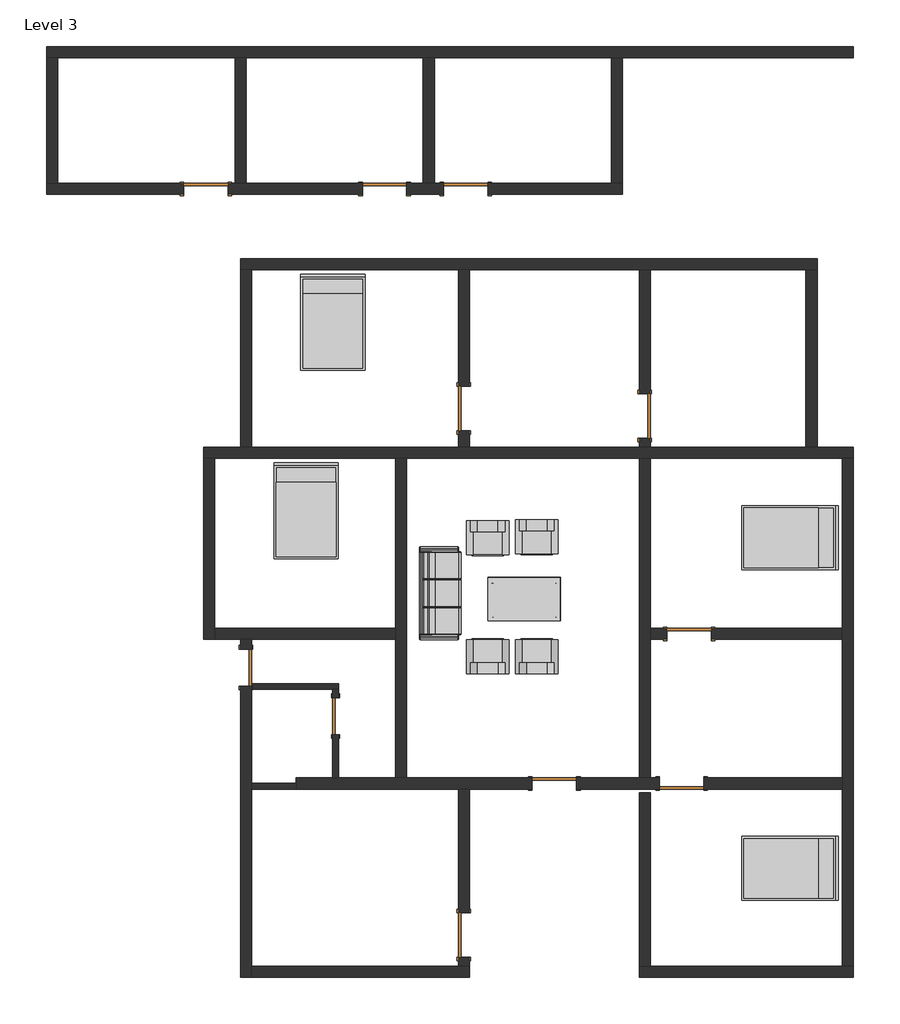
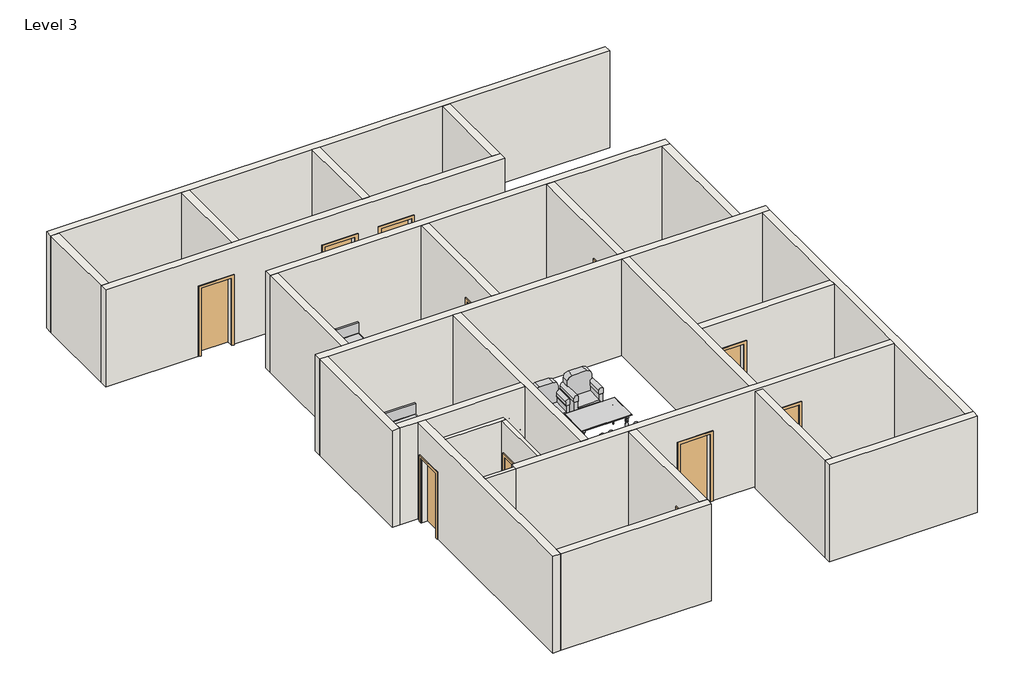
# One storey, incomplete: 27 walls, 11 doors, 10 furniture elements.
"""IFC4 building model written with IfcOpenShell, lengths in millimetres."""

from ifc_helpers import new_model, si_unit, frame, origin, place, context, project, spatial, polyline, outline, extrude, faceted_brep, transform, mapped, element, save
from components import door_a1484949, door_d8f5dbb5, door_0ca8825f, door_a90ba1ad, furniture_2fc85b74, furniture_29a9adb8, furniture_57072a26, bed_17739_bed_17739_15c61121, chair_lounge_11461_couch_0866092f, dining_table_14755_dining_table_14755_d89cb775

model = new_model("IFC4")

# Units and contexts
model_context = context("Model", 3, world=origin())
ifc_project = project(units=[si_unit("LENGTHUNIT", "METRE", prefix="MILLI")], contexts=[model_context])

# Site, building, storey
site = spatial("IfcSite", under=ifc_project)
building = spatial("IfcBuilding", under=site)
storey = spatial("IfcBuildingStorey", under=building, Name="Level 3", Elevation=3200.4)

# Doors
placement = place(None, origin())
door_shape = door_a1484949(model_context)
element("IfcDoor", 1, ObjectType="Single-Flush : 30\" x 80\"", at=placement, inside=storey, context=model_context, shape_type="MappedRepresentation", body=[
    mapped(door_shape, transform((-6124.8057305, -546.3292186, 3200.4), x_axis=(0.0, -1.0, 0.0), y_axis=(1.0, 0.0, 0.0), z_axis=(0.0, 0.0, 1.0))),
])
door_2_shape = door_d8f5dbb5(model_context)
element("IfcDoor", 2, ObjectType="Single-Flush : 30\" x 80\"", at=placement, inside=storey, context=model_context, shape_type="MappedRepresentation", body=[
    mapped(door_2_shape, transform((-4276.442132, -1546.4542186, 3200.4), x_axis=(0.0, 1.0, 0.0), y_axis=(-1.0, 0.0, 0.0), z_axis=(0.0, 0.0, 1.0))),
])
door_3_shape = door_0ca8825f(model_context)
element("IfcDoor", 3, ObjectType="Single-Flush : 36\" x 84\"", at=placement, inside=storey, context=model_context, shape_type="MappedRepresentation", body=[
    mapped(door_3_shape, transform((-6952.8959326, 9329.2722985, 3200.4), x_axis=(1.0, 0.0, 0.0), y_axis=(0.0, 1.0, 0.0), z_axis=(0.0, 0.0, 1.0))),
])
element("IfcDoor", 4, ObjectType="Single-Flush : 36\" x 84\"", at=placement, inside=storey, context=model_context, shape_type="MappedRepresentation", body=[
    mapped(door_3_shape, transform((-3267.5476203, 9329.2722985, 3200.4), x_axis=(1.0, 0.0, 0.0), y_axis=(0.0, 1.0, 0.0), z_axis=(0.0, 0.0, 1.0))),
])
element("IfcDoor", 5, ObjectType="Single-Flush : 36\" x 84\"", at=placement, inside=storey, context=model_context, shape_type="MappedRepresentation", body=[
    mapped(door_3_shape, transform((2105.307868, 4644.7957814, 3200.4), x_axis=(0.0, -1.0, 0.0), y_axis=(1.0, 0.0, 0.0), z_axis=(0.0, 0.0, 1.0))),
])
element("IfcDoor", 6, ObjectType="Single-Flush : 36\" x 84\"", at=placement, inside=storey, context=model_context, shape_type="MappedRepresentation", body=[
    mapped(door_3_shape, transform((2867.307868, -2937.1042186, 3200.4), x_axis=(-1.0, 0.0, 0.0), y_axis=(0.0, -1.0, 0.0), z_axis=(0.0, 0.0, 1.0))),
])
element("IfcDoor", 7, ObjectType="Single-Flush : 36\" x 84\"", at=placement, inside=storey, context=model_context, shape_type="MappedRepresentation", body=[
    mapped(door_3_shape, transform((238.407868, -2937.1042186, 3200.4), x_axis=(1.0, 0.0, 0.0), y_axis=(0.0, 1.0, 0.0), z_axis=(0.0, 0.0, 1.0))),
])
door_4_shape = door_a90ba1ad(model_context)
element("IfcDoor", 8, ObjectType="Single-Flush : 36\" x 84\"", at=placement, inside=storey, context=model_context, shape_type="MappedRepresentation", body=[
    mapped(door_4_shape, transform((-1591.1476203, 9329.2722985, 3200.4), x_axis=(-1.0, 0.0, 0.0), y_axis=(0.0, -1.0, 0.0), z_axis=(0.0, 0.0, 1.0))),
])
element("IfcDoor", 9, ObjectType="Single-Flush : 36\" x 84\"", at=placement, inside=storey, context=model_context, shape_type="MappedRepresentation", body=[
    mapped(door_4_shape, transform((-1628.492132, 4797.1957814, 3200.4), x_axis=(0.0, -1.0, 0.0), y_axis=(1.0, 0.0, 0.0), z_axis=(0.0, 0.0, 1.0))),
])
element("IfcDoor", 10, ObjectType="Single-Flush : 36\" x 84\"", at=placement, inside=storey, context=model_context, shape_type="MappedRepresentation", body=[
    mapped(door_4_shape, transform((3019.707868, 148.9957814, 3200.4), x_axis=(-1.0, 0.0, 0.0), y_axis=(0.0, -1.0, 0.0), z_axis=(0.0, 0.0, 1.0))),
])
element("IfcDoor", 11, ObjectType="Single-Flush : 36\" x 84\"", at=placement, inside=storey, context=model_context, shape_type="MappedRepresentation", body=[
    mapped(door_4_shape, transform((-1628.492132, -6061.3042186, 3200.4), x_axis=(0.0, -1.0, 0.0), y_axis=(1.0, 0.0, 0.0), z_axis=(0.0, 0.0, 1.0))),
])

# Furniture
furniture_shape = furniture_2fc85b74(model_context)
furniture_2_shape = furniture_29a9adb8(model_context)
furniture_3_shape = furniture_57072a26(model_context)
element("IfcFurniture", 12, at=placement, inside=storey, context=model_context, shape_type="MappedRepresentation", body=[
    mapped(furniture_shape, transform((-1742.792132, 987.1957814, 3200.4), x_axis=(0.0, 1.0, 0.0), y_axis=(-1.0, 0.0, 0.0), z_axis=(0.0, 0.0, 1.0))),
    mapped(furniture_2_shape, transform((-1742.792132, 987.1957814, 3200.4), x_axis=(0.0, 1.0, 0.0), y_axis=(-1.0, 0.0, 0.0), z_axis=(0.0, 0.0, 1.0))),
    mapped(furniture_3_shape, transform((-1742.792132, 987.1957814, 3200.4), x_axis=(0.0, 1.0, 0.0), y_axis=(-1.0, 0.0, 0.0), z_axis=(0.0, 0.0, 1.0))),
])
bed_17739_bed_17739_shape = bed_17739_bed_17739_15c61121(model_context)
element("IfcFurniture", 13, ObjectType="Bed_17739 : Bed_17739", at=placement, inside=storey, context=model_context, shape_type="MappedRepresentation", body=[
    mapped(bed_17739_bed_17739_shape, transform((-4333.592132, 6549.7957814, 3200.4), x_axis=(1.0, 0.0, 0.0), y_axis=(0.0, 1.0, 0.0), z_axis=(0.0, 0.0, 1.0))),
])
element("IfcFurniture", 14, ObjectType="Bed_17739 : Bed_17739", at=placement, inside=storey, context=model_context, shape_type="MappedRepresentation", body=[
    mapped(bed_17739_bed_17739_shape, transform((5077.107868, 2130.1957814, 3200.4), x_axis=(0.0, -1.0, 0.0), y_axis=(1.0, 0.0, 0.0), z_axis=(0.0, 0.0, 1.0))),
])
element("IfcFurniture", 15, ObjectType="Bed_17739 : Bed_17739", at=placement, inside=storey, context=model_context, shape_type="MappedRepresentation", body=[
    mapped(bed_17739_bed_17739_shape, transform((5077.107868, -4689.7042186, 3200.4), x_axis=(0.0, -1.0, 0.0), y_axis=(1.0, 0.0, 0.0), z_axis=(0.0, 0.0, 1.0))),
])
element("IfcFurniture", 16, ObjectType="Bed_17739 : Bed_17739", at=placement, inside=storey, context=model_context, shape_type="MappedRepresentation", body=[
    mapped(bed_17739_bed_17739_shape, transform((-4886.042132, 2663.5957814, 3200.4), x_axis=(1.0, 0.0, 0.0), y_axis=(0.0, 1.0, 0.0), z_axis=(0.0, 0.0, 1.0))),
])
chair_lounge_11461_couch_shape = chair_lounge_11461_couch_0866092f(model_context)
element("IfcFurniture", 17, ObjectType="Chair-Lounge_11461 : Couch", at=placement, inside=storey, context=model_context, shape_type="MappedRepresentation", body=[
    mapped(chair_lounge_11461_couch_shape, transform((-1135.6501746, 2478.1239494, 3200.4), x_axis=(1.0, 0.0, 0.0), y_axis=(0.0, 1.0, 0.0), z_axis=(0.0, 0.0, 1.0))),
])
element("IfcFurniture", 18, ObjectType="Chair-Lounge_11461 : Couch", at=placement, inside=storey, context=model_context, shape_type="MappedRepresentation", body=[
    mapped(chair_lounge_11461_couch_shape, transform((-1135.6501746, -676.3685812, 3200.4), x_axis=(-1.0, 0.0, 0.0), y_axis=(0.0, -1.0, 0.0), z_axis=(0.0, 0.0, 1.0))),
])
element("IfcFurniture", 19, ObjectType="Chair-Lounge_11461 : Couch", at=placement, inside=storey, context=model_context, shape_type="MappedRepresentation", body=[
    mapped(chair_lounge_11461_couch_shape, transform((-125.9107827, -676.3685812, 3200.4), x_axis=(-1.0, 0.0, 0.0), y_axis=(0.0, -1.0, 0.0), z_axis=(0.0, 0.0, 1.0))),
])
element("IfcFurniture", 20, ObjectType="Chair-Lounge_11461 : Couch", at=placement, inside=storey, context=model_context, shape_type="MappedRepresentation", body=[
    mapped(chair_lounge_11461_couch_shape, transform((-125.9107827, 2504.7969663, 3200.4), x_axis=(1.0, 0.0, 0.0), y_axis=(0.0, 1.0, 0.0), z_axis=(0.0, 0.0, 1.0))),
])
dining_table_14755_dining_table_14755_shape = dining_table_14755_dining_table_14755_d89cb775(model_context)
element("IfcFurniture", 21, ObjectType="Dining_table_14755 : Dining_table_14755", at=placement, inside=storey, context=model_context, shape_type="MappedRepresentation", body=[
    mapped(dining_table_14755_dining_table_14755_shape, transform((-1135.6501746, 415.6957814, 3200.4), x_axis=(1.0, 0.0, 0.0), y_axis=(0.0, 1.0, 0.0), z_axis=(0.0, 0.0, 1.0))),
])

# Walls
element("IfcWall", 22, ObjectType="4.5\"WALL", at=placement, inside=storey, context=model_context, shape_type="Brep", body=[
    faceted_brep([(-6010.5057305, -994.0042186, 3200.4), (-4333.592132, -994.0042186, 3200.4), (-4219.292132, -994.0042186, 3200.4), (-4219.292132, -994.0042186, 6248.4), (-4333.592132, -994.0042186, 6248.4), (-6010.5057305, -994.0042186, 6248.4), (-6010.5057305, -879.7042186, 3200.4), (-6010.5057305, -879.7042186, 6248.4), (-4219.292132, -879.7042186, 6248.4), (-4219.292132, -879.7042186, 3200.4)], [[[0, 1, 2, 3, 4, 5]], [[6, 7, 8, 9]], [[2, 1, 0, 6, 9]], [[0, 5, 7, 6]], [[3, 2, 9, 8]], [[5, 4, 3, 8, 7]]]),
])
element("IfcWall", 23, ObjectType="4.5\"WALL", at=placement, inside=storey, context=model_context, shape_type="SweptSolid", body=[
    extrude(outline(polyline([(-994.0042186, 3200.4), (-1165.4542186, 3200.4), (-1165.4542186, 5232.4), (-1927.4542186, 5232.4), (-1927.4542186, 3200.4), (-2822.8042186, 3200.4), (-2822.8042186, 6248.4), (-994.0042186, 6248.4), (-994.0042186, 3200.4)])), frame((-4333.592132, 0.0, 0.0), z_axis=(1.0, 0.0, 0.0), x_axis=(0.0, 1.0, 0.0)), (0.0, 0.0, 1.0), 114.3),
])
element("IfcWall", 24, ObjectType="4.5\"WALL", at=placement, inside=storey, context=model_context, shape_type="SweptSolid", body=[
    extrude(outline(polyline([(-5096.0236102, -3051.4042186), (-6010.5057305, -3051.4042186), (-6010.5057305, -2937.1042186), (-5096.0236102, -2937.1042186), (-5096.0236102, -3051.4042186)])), frame((0.0, 0.0, 3200.4), z_axis=(0.0, 0.0, 1.0), x_axis=(1.0, 0.0, 0.0)), (0.0, 0.0, 1.0), 3048.0),
])
element("IfcWall", 25, ObjectType="WALL9\"", at=placement, inside=storey, context=model_context, shape_type="Brep", body=[
    faceted_brep([(-10239.8476203, 12034.3722985, 3200.4), (-10011.2476203, 12034.3722985, 3200.4), (-6353.6476203, 12034.3722985, 3200.4), (-6125.0476203, 12034.3722985, 3200.4), (-2467.4476203, 12034.3722985, 3200.4), (-2238.8476203, 12034.3722985, 3200.4), (1418.7523797, 12034.3722985, 3200.4), (1647.3523797, 12034.3722985, 3200.4), (6410.607868, 12034.3722985, 3200.4), (6410.607868, 12034.3722985, 6248.4), (1647.3523797, 12034.3722985, 6248.4), (1418.7523797, 12034.3722985, 6248.4), (-2238.8476203, 12034.3722985, 6248.4), (-2467.4476203, 12034.3722985, 6248.4), (-6125.0476203, 12034.3722985, 6248.4), (-6353.6476203, 12034.3722985, 6248.4), (-10011.2476203, 12034.3722985, 6248.4), (-10239.8476203, 12034.3722985, 6248.4), (-10239.8476203, 12262.9722985, 3200.4), (-10239.8476203, 12262.9722985, 6248.4), (6410.607868, 12262.9722985, 6248.4), (6410.607868, 12262.9722985, 3200.4)], [[[0, 1, 2, 3, 4, 5, 6, 7, 8, 9, 10, 11, 12, 13, 14, 15, 16, 17]], [[18, 19, 20, 21]], [[8, 7, 6, 5, 4, 3, 2, 1, 0, 18, 21]], [[9, 8, 21, 20]], [[17, 16, 15, 14, 13, 12, 11, 10, 9, 20, 19]], [[0, 17, 19, 18]]]),
])
element("IfcWall", 26, ObjectType="WALL9\"", at=placement, inside=storey, context=model_context, shape_type="Brep", body=[
    faceted_brep([(-2810.3476203, 9214.9722985, 3200.4), (-2048.3476203, 9214.9722985, 3200.4), (-2048.3476203, 9214.9722985, 5334.0), (-1133.9476203, 9214.9722985, 5334.0), (-1133.9476203, 9214.9722985, 3200.4), (1647.3523797, 9214.9722985, 3200.4), (1647.3523797, 9214.9722985, 6248.4), (-6238.592132, 9214.9722985, 6248.4), (-10241.6673123, 9214.9722985, 6248.4), (-10241.6673123, 9214.9722985, 3200.4), (-7410.0959326, 9214.9722985, 3200.4), (-7410.0959326, 9214.9722985, 5334.0), (-6495.6959326, 9214.9722985, 5334.0), (-6495.6959326, 9214.9722985, 3200.4), (-3724.7476203, 9214.9722985, 3200.4), (-3724.7476203, 9214.9722985, 5334.0), (-2810.3476203, 9214.9722985, 5334.0), (-2048.3476203, 9443.5722985, 5334.0), (-2048.3476203, 9443.5722985, 3200.4), (-2238.8476203, 9443.5722985, 3200.4), (-2467.4476203, 9443.5722985, 3200.4), (-2810.3476203, 9443.5722985, 3200.4), (-2810.3476203, 9443.5722985, 5334.0), (-3724.7476203, 9443.5722985, 5334.0), (-3724.7476203, 9443.5722985, 3200.4), (-6125.0476203, 9443.5722985, 3200.4), (-6353.6476203, 9443.5722985, 3200.4), (-6495.6959326, 9443.5722985, 3200.4), (-6495.6959326, 9443.5722985, 5334.0), (-7410.0959326, 9443.5722985, 5334.0), (-7410.0959326, 9443.5722985, 3200.4), (-10011.2476203, 9443.5722985, 3200.4), (-10239.8476203, 9443.5722985, 3200.4), (-10241.6673123, 9443.5722985, 3200.4), (-10241.6673123, 9443.5722985, 6248.4), (-10239.8476203, 9443.5722985, 6248.4), (-10011.2476203, 9443.5722985, 6248.4), (-6353.6476203, 9443.5722985, 6248.4), (-6125.0476203, 9443.5722985, 6248.4), (-2467.4476203, 9443.5722985, 6248.4), (-2238.8476203, 9443.5722985, 6248.4), (1418.7523797, 9443.5722985, 6248.4), (1647.3523797, 9443.5722985, 6248.4), (1647.3523797, 9443.5722985, 3200.4), (1418.7523797, 9443.5722985, 3200.4), (-1133.9476203, 9443.5722985, 3200.4), (-1133.9476203, 9443.5722985, 5334.0)], [[[0, 1, 2, 3, 4, 5, 6, 7, 8, 9, 10, 11, 12, 13, 14, 15, 16]], [[17, 18, 19, 20, 21, 22, 23, 24, 25, 26, 27, 28, 29, 30, 31, 32, 33, 34, 35, 36, 37, 38, 39, 40, 41, 42, 43, 44, 45, 46]], [[10, 9, 33, 32, 31, 30]], [[14, 13, 27, 26, 25, 24]], [[45, 44, 43, 5, 4]], [[21, 20, 19, 18, 1, 0]], [[9, 8, 34, 33]], [[6, 5, 43, 42]], [[28, 27, 13, 12]], [[29, 28, 12, 11]], [[30, 29, 11, 10]], [[22, 21, 0, 16]], [[23, 22, 16, 15]], [[24, 23, 15, 14]], [[2, 1, 18, 17]], [[3, 2, 17, 46]], [[4, 3, 46, 45]], [[8, 7, 6, 42, 41, 40, 39, 38, 37, 36, 35, 34]]]),
])
element("IfcWall", 27, ObjectType="WALL9\"", at=placement, inside=storey, context=model_context, shape_type="SweptSolid", body=[
    extrude(outline(polyline([(1647.3523797, 12034.3722985), (1647.3523797, 9443.5722985), (1418.7523797, 9443.5722985), (1418.7523797, 12034.3722985), (1647.3523797, 12034.3722985)])), frame((0.0, 0.0, 3200.4), z_axis=(0.0, 0.0, 1.0), x_axis=(1.0, 0.0, 0.0)), (0.0, 0.0, 1.0), 3048.0),
])
element("IfcWall", 28, ObjectType="WALL9\"", at=placement, inside=storey, context=model_context, shape_type="SweptSolid", body=[
    extrude(outline(polyline([(-2467.4476203, 9443.5722985), (-2467.4476203, 12034.3722985), (-2238.8476203, 12034.3722985), (-2238.8476203, 9443.5722985), (-2467.4476203, 9443.5722985)])), frame((0.0, 0.0, 3200.4), z_axis=(0.0, 0.0, 1.0), x_axis=(1.0, 0.0, 0.0)), (0.0, 0.0, 1.0), 3048.0),
])
element("IfcWall", 29, ObjectType="WALL9\"", at=placement, inside=storey, context=model_context, shape_type="SweptSolid", body=[
    extrude(outline(polyline([(-6353.6476203, 9443.5722985), (-6353.6476203, 12034.3722985), (-6125.0476203, 12034.3722985), (-6125.0476203, 9443.5722985), (-6353.6476203, 9443.5722985)])), frame((0.0, 0.0, 3200.4), z_axis=(0.0, 0.0, 1.0), x_axis=(1.0, 0.0, 0.0)), (0.0, 0.0, 1.0), 3048.0),
])
element("IfcWall", 30, ObjectType="WALL9\"", at=placement, inside=storey, context=model_context, shape_type="Brep", body=[
    faceted_brep([(-6238.592132, 7654.6957814, 3200.4), (-6009.992132, 7654.6957814, 3200.4), (-1742.792132, 7654.6957814, 3200.4), (-1514.192132, 7654.6957814, 3200.4), (1991.007868, 7654.6957814, 3200.4), (2219.607868, 7654.6957814, 3200.4), (5432.707868, 7654.6957814, 3200.4), (5661.307868, 7654.6957814, 3200.4), (5661.307868, 7654.6957814, 6248.4), (5432.707868, 7654.6957814, 6248.4), (2219.607868, 7654.6957814, 6248.4), (1991.007868, 7654.6957814, 6248.4), (-1514.192132, 7654.6957814, 6248.4), (-1742.792132, 7654.6957814, 6248.4), (-6009.992132, 7654.6957814, 6248.4), (-6238.592132, 7654.6957814, 6248.4), (-6238.592132, 7883.2957814, 3200.4), (-6238.592132, 7883.2957814, 6248.4), (5661.307868, 7883.2957814, 6248.4), (5661.307868, 7883.2957814, 3200.4)], [[[0, 1, 2, 3, 4, 5, 6, 7, 8, 9, 10, 11, 12, 13, 14, 15]], [[16, 17, 18, 19]], [[7, 6, 5, 4, 3, 2, 1, 0, 16, 19]], [[0, 15, 17, 16]], [[15, 14, 13, 12, 11, 10, 9, 8, 18, 17]], [[8, 7, 19, 18]]]),
])
element("IfcWall", 31, ObjectType="WALL9\"", at=placement, inside=storey, context=model_context, shape_type="SweptSolid", body=[
    extrude(outline(polyline([(-6238.592132, 3997.0957814), (-6238.592132, 7654.6957814), (-6009.992132, 7654.6957814), (-6009.992132, 3997.0957814), (-6238.592132, 3997.0957814)])), frame((0.0, 0.0, 3200.4), z_axis=(0.0, 0.0, 1.0), x_axis=(1.0, 0.0, 0.0)), (0.0, 0.0, 1.0), 3048.0),
])
element("IfcWall", 32, ObjectType="WALL9\"", at=placement, inside=storey, context=model_context, shape_type="SweptSolid", body=[
    extrude(outline(polyline([(4339.9957814, 5334.0), (4339.9957814, 3200.4), (3997.0957814, 3200.4), (3997.0957814, 6248.4), (7654.6957814, 6248.4), (7654.6957814, 3200.4), (5254.3957814, 3200.4), (5254.3957814, 5334.0), (4339.9957814, 5334.0)])), frame((-1742.792132, 0.0, 0.0), z_axis=(1.0, 0.0, 0.0), x_axis=(0.0, 1.0, 0.0)), (0.0, 0.0, 1.0), 228.6),
])
element("IfcWall", 33, ObjectType="WALL9\"", at=placement, inside=storey, context=model_context, shape_type="SweptSolid", body=[
    extrude(outline(polyline([(4187.5957814, 5334.0), (4187.5957814, 3200.4), (3997.0957814, 3200.4), (3997.0957814, 6248.4), (7654.6957814, 6248.4), (7654.6957814, 3200.4), (5101.9957814, 3200.4), (5101.9957814, 5334.0), (4187.5957814, 5334.0)])), frame((1991.007868, 0.0, 0.0), z_axis=(1.0, 0.0, 0.0), x_axis=(0.0, 1.0, 0.0)), (0.0, 0.0, 1.0), 228.6),
])
element("IfcWall", 34, ObjectType="WALL9\"", at=placement, inside=storey, context=model_context, shape_type="Brep", body=[
    faceted_brep([(-7000.592132, 3768.4957814, 3200.4), (-6771.992132, 3768.4957814, 3200.4), (-3038.192132, 3768.4957814, 3200.4), (-2809.592132, 3768.4957814, 3200.4), (1991.007868, 3768.4957814, 3200.4), (2219.607868, 3768.4957814, 3200.4), (6182.007868, 3768.4957814, 3200.4), (6410.607868, 3768.4957814, 3200.4), (6410.607868, 3768.4957814, 6248.4), (6182.007868, 3768.4957814, 6248.4), (2219.607868, 3768.4957814, 6248.4), (1991.007868, 3768.4957814, 6248.4), (-2809.592132, 3768.4957814, 6248.4), (-3038.192132, 3768.4957814, 6248.4), (-6771.992132, 3768.4957814, 6248.4), (-7000.592132, 3768.4957814, 6248.4), (-7000.592132, 3997.0957814, 3200.4), (-7000.592132, 3997.0957814, 6248.4), (-6238.592132, 3997.0957814, 6248.4), (-6009.992132, 3997.0957814, 6248.4), (-1742.792132, 3997.0957814, 6248.4), (-1514.192132, 3997.0957814, 6248.4), (1991.007868, 3997.0957814, 6248.4), (2219.607868, 3997.0957814, 6248.4), (5432.707868, 3997.0957814, 6248.4), (5661.307868, 3997.0957814, 6248.4), (6410.607868, 3997.0957814, 6248.4), (6410.607868, 3997.0957814, 3200.4), (5661.307868, 3997.0957814, 3200.4), (5432.707868, 3997.0957814, 3200.4), (2219.607868, 3997.0957814, 3200.4), (1991.007868, 3997.0957814, 3200.4), (-1514.192132, 3997.0957814, 3200.4), (-1742.792132, 3997.0957814, 3200.4), (-6009.992132, 3997.0957814, 3200.4), (-6238.592132, 3997.0957814, 3200.4)], [[[0, 1, 2, 3, 4, 5, 6, 7, 8, 9, 10, 11, 12, 13, 14, 15]], [[16, 17, 18, 19, 20, 21, 22, 23, 24, 25, 26, 27, 28, 29, 30, 31, 32, 33, 34, 35]], [[7, 6, 5, 4, 3, 2, 1, 0, 16, 35, 34, 33, 32, 31, 30, 29, 28, 27]], [[0, 15, 17, 16]], [[15, 14, 13, 12, 11, 10, 9, 8, 26, 25, 24, 23, 22, 21, 20, 19, 18, 17]], [[8, 7, 27, 26]]]),
])
element("IfcWall", 35, ObjectType="WALL9\"", at=placement, inside=storey, context=model_context, shape_type="SweptSolid", body=[
    extrude(outline(polyline([(3200.4, 2219.607868), (3200.4, 2562.507868), (5334.0, 2562.507868), (5334.0, 3476.907868), (3200.4, 3476.907868), (3200.4, 6182.007868), (6248.4, 6182.007868), (6248.4, 2219.607868), (3200.4, 2219.607868)])), frame((0.0, 34.6957814, 0.0), z_axis=(0.0, 1.0, 0.0), x_axis=(0.0, 0.0, 1.0)), (0.0, 0.0, 1.0), 228.6),
])
element("IfcWall", 36, ObjectType="WALL9\"", at=placement, inside=storey, context=model_context, shape_type="Brep", body=[
    faceted_brep([(-7000.592132, 3768.4957814, 3200.4), (-7000.592132, 34.6957814, 3200.4), (-7000.592132, 34.6957814, 6248.4), (-7000.592132, 3768.4957814, 6248.4), (-6771.992132, 3768.4957814, 3200.4), (-6771.992132, 3768.4957814, 6248.4), (-6771.992132, 263.2957814, 6248.4), (-6771.992132, 34.6957814, 6248.4), (-6771.992132, 34.6957814, 3200.4), (-6771.992132, 263.2957814, 3200.4)], [[[0, 1, 2, 3]], [[4, 5, 6, 7, 8, 9]], [[1, 0, 4, 9, 8]], [[0, 3, 5, 4]], [[2, 1, 8, 7]], [[3, 2, 7, 6, 5]]]),
])
element("IfcWall", 37, ObjectType="WALL9\"", at=placement, inside=storey, context=model_context, shape_type="Brep", body=[
    faceted_brep([(-6771.992132, 34.6957814, 3200.4), (-6239.1057305, 34.6957814, 3200.4), (-6010.5057305, 34.6957814, 3200.4), (-3038.192132, 34.6957814, 3200.4), (-3038.192132, 34.6957814, 6248.4), (-6010.5057305, 34.6957814, 6248.4), (-6239.1057305, 34.6957814, 6248.4), (-6771.992132, 34.6957814, 6248.4), (-6771.992132, 263.2957814, 3200.4), (-6771.992132, 263.2957814, 6248.4), (-3038.192132, 263.2957814, 6248.4), (-3038.192132, 263.2957814, 3200.4)], [[[0, 1, 2, 3, 4, 5, 6, 7]], [[8, 9, 10, 11]], [[3, 2, 1, 0, 8, 11]], [[0, 7, 9, 8]], [[4, 3, 11, 10]], [[7, 6, 5, 4, 10, 9]]]),
])
element("IfcWall", 38, ObjectType="WALL9\"", at=placement, inside=storey, context=model_context, shape_type="Brep", body=[
    faceted_brep([(-3038.192132, 3768.4957814, 3200.4), (-3038.192132, 263.2957814, 3200.4), (-3038.192132, 34.6957814, 3200.4), (-3038.192132, -2822.8042186, 3200.4), (-3038.192132, -2822.8042186, 6248.4), (-3038.192132, 34.6957814, 6248.4), (-3038.192132, 263.2957814, 6248.4), (-3038.192132, 3768.4957814, 6248.4), (-2809.592132, 3768.4957814, 3200.4), (-2809.592132, 3768.4957814, 6248.4), (-2809.592132, -2822.8042186, 6248.4), (-2809.592132, -2822.8042186, 3200.4)], [[[0, 1, 2, 3, 4, 5, 6, 7]], [[8, 9, 10, 11]], [[3, 2, 1, 0, 8, 11]], [[0, 7, 9, 8]], [[4, 3, 11, 10]], [[7, 6, 5, 4, 10, 9]]]),
])
element("IfcWall", 39, ObjectType="WALL9\"", at=placement, inside=storey, context=model_context, shape_type="Brep", body=[
    faceted_brep([(1991.007868, 3768.4957814, 3200.4), (1991.007868, -2822.8042186, 3200.4), (1991.007868, -2822.8042186, 6248.4), (1991.007868, 3768.4957814, 6248.4), (2219.607868, 3768.4957814, 3200.4), (2219.607868, 3768.4957814, 6248.4), (2219.607868, 263.2957814, 6248.4), (2219.607868, 34.6957814, 6248.4), (2219.607868, -2822.8042186, 6248.4), (2219.607868, -2822.8042186, 3200.4), (2219.607868, 34.6957814, 3200.4), (2219.607868, 263.2957814, 3200.4)], [[[0, 1, 2, 3]], [[4, 5, 6, 7, 8, 9, 10, 11]], [[1, 0, 4, 11, 10, 9]], [[0, 3, 5, 4]], [[2, 1, 9, 8]], [[3, 2, 8, 7, 6, 5]]]),
])
element("IfcWall", 40, ObjectType="WALL9\"", at=placement, inside=storey, context=model_context, shape_type="Brep", body=[
    faceted_brep([(-6239.1057305, -927.3292186, 5232.4), (-6239.1057305, -927.3292186, 3200.4), (-6239.1057305, -6937.6042186, 3200.4), (-6239.1057305, -6937.6042186, 6248.4), (-6239.1057305, 34.6957814, 6248.4), (-6239.1057305, 34.6957814, 3200.4), (-6239.1057305, -165.3292186, 3200.4), (-6239.1057305, -165.3292186, 5232.4), (-6010.5057305, -6937.6042186, 3200.4), (-6010.5057305, -6709.0042186, 3200.4), (-6010.5057305, -3051.4042186, 3200.4), (-6010.5057305, -2937.1042186, 3200.4), (-6010.5057305, -994.0042186, 3200.4), (-6010.5057305, -927.3292186, 3200.4), (-6010.5057305, -927.3292186, 5232.4), (-6010.5057305, -165.3292186, 5232.4), (-6010.5057305, -165.3292186, 3200.4), (-6010.5057305, 34.6957814, 3200.4), (-6010.5057305, 34.6957814, 6248.4), (-6010.5057305, -879.7042186, 6248.4), (-6010.5057305, -994.0042186, 6248.4), (-6010.5057305, -2937.1042186, 6248.4), (-6010.5057305, -3051.4042186, 6248.4), (-6010.5057305, -6709.0042186, 6248.4), (-6010.5057305, -6937.6042186, 6248.4)], [[[0, 1, 2, 3, 4, 5, 6, 7]], [[8, 9, 10, 11, 12, 13, 14, 15, 16, 17, 18, 19, 20, 21, 22, 23, 24]], [[6, 5, 17, 16]], [[2, 1, 13, 12, 11, 10, 9, 8]], [[5, 4, 18, 17]], [[3, 2, 8, 24]], [[14, 13, 1, 0]], [[15, 14, 0, 7]], [[16, 15, 7, 6]], [[4, 3, 24, 23, 22, 21, 20, 19, 18]]]),
])
element("IfcWall", 41, ObjectType="WALL9\"", at=placement, inside=storey, context=model_context, shape_type="Brep", body=[
    faceted_brep([(-1514.192132, -6709.0042186, 3200.4), (-1742.792132, -6709.0042186, 3200.4), (-6010.5057305, -6709.0042186, 3200.4), (-6010.5057305, -6709.0042186, 6248.4), (-1742.792132, -6709.0042186, 6248.4), (-1514.192132, -6709.0042186, 6248.4), (-1514.192132, -6937.6042186, 3200.4), (-1514.192132, -6937.6042186, 6248.4), (-6010.5057305, -6937.6042186, 6248.4), (-6010.5057305, -6937.6042186, 3200.4)], [[[0, 1, 2, 3, 4, 5]], [[6, 7, 8, 9]], [[2, 1, 0, 6, 9]], [[3, 2, 9, 8]], [[0, 5, 7, 6]], [[5, 4, 3, 8, 7]]]),
])
element("IfcWall", 42, ObjectType="WALL9\"", at=placement, inside=storey, context=model_context, shape_type="Brep", body=[
    faceted_brep([(695.607868, -3051.4042186, 5334.0), (695.607868, -3051.4042186, 3200.4), (2410.107868, -3051.4042186, 3200.4), (2410.107868, -3051.4042186, 5334.0), (3324.507868, -3051.4042186, 5334.0), (3324.507868, -3051.4042186, 3200.4), (6182.007868, -3051.4042186, 3200.4), (6182.007868, -3051.4042186, 6248.4), (-1514.192132, -3051.4042186, 6248.4), (-1742.792132, -3051.4042186, 6248.4), (-5096.0236102, -3051.4042186, 6248.4), (-5096.0236102, -3051.4042186, 3200.4), (-1742.792132, -3051.4042186, 3200.4), (-1514.192132, -3051.4042186, 3200.4), (-218.792132, -3051.4042186, 3200.4), (-218.792132, -3051.4042186, 5334.0), (2410.107868, -2822.8042186, 3200.4), (2219.607868, -2822.8042186, 3200.4), (1991.007868, -2822.8042186, 3200.4), (695.607868, -2822.8042186, 3200.4), (695.607868, -2822.8042186, 5334.0), (-218.792132, -2822.8042186, 5334.0), (-218.792132, -2822.8042186, 3200.4), (-2809.592132, -2822.8042186, 3200.4), (-3038.192132, -2822.8042186, 3200.4), (-4219.292132, -2822.8042186, 3200.4), (-4333.592132, -2822.8042186, 3200.4), (-5096.0236102, -2822.8042186, 3200.4), (-5096.0236102, -2822.8042186, 6248.4), (-4333.592132, -2822.8042186, 6248.4), (-4219.292132, -2822.8042186, 6248.4), (-3038.192132, -2822.8042186, 6248.4), (-2809.592132, -2822.8042186, 6248.4), (1991.007868, -2822.8042186, 6248.4), (2219.607868, -2822.8042186, 6248.4), (6182.007868, -2822.8042186, 6248.4), (6182.007868, -2822.8042186, 3200.4), (3324.507868, -2822.8042186, 3200.4), (3324.507868, -2822.8042186, 5334.0), (2410.107868, -2822.8042186, 5334.0), (-5096.0236102, -2937.1042186, 3200.4), (-5096.0236102, -2937.1042186, 6248.4)], [[[0, 1, 2, 3, 4, 5, 6, 7, 8, 9, 10, 11, 12, 13, 14, 15]], [[16, 17, 18, 19, 20, 21, 22, 23, 24, 25, 26, 27, 28, 29, 30, 31, 32, 33, 34, 35, 36, 37, 38, 39]], [[37, 36, 6, 5]], [[2, 1, 19, 18, 17, 16]], [[14, 13, 12, 11, 40, 27, 26, 25, 24, 23, 22]], [[11, 10, 41, 28, 27, 40]], [[3, 2, 16, 39]], [[4, 3, 39, 38]], [[5, 4, 38, 37]], [[20, 19, 1, 0]], [[21, 20, 0, 15]], [[22, 21, 15, 14]], [[10, 9, 8, 7, 35, 34, 33, 32, 31, 30, 29, 28, 41]], [[7, 6, 36, 35]]]),
])
element("IfcWall", 43, ObjectType="WALL9\"", at=placement, inside=storey, context=model_context, shape_type="Brep", body=[
    faceted_brep([(6410.607868, -6709.0042186, 3200.4), (6182.007868, -6709.0042186, 3200.4), (2219.607868, -6709.0042186, 3200.4), (1991.007868, -6709.0042186, 3200.4), (1991.007868, -6709.0042186, 6248.4), (2219.607868, -6709.0042186, 6248.4), (6182.007868, -6709.0042186, 6248.4), (6410.607868, -6709.0042186, 6248.4), (6410.607868, -6937.6042186, 3200.4), (6410.607868, -6937.6042186, 6248.4), (1991.007868, -6937.6042186, 6248.4), (1991.007868, -6937.6042186, 3200.4)], [[[0, 1, 2, 3, 4, 5, 6, 7]], [[8, 9, 10, 11]], [[3, 2, 1, 0, 8, 11]], [[4, 3, 11, 10]], [[7, 6, 5, 4, 10, 9]], [[0, 7, 9, 8]]]),
])
element("IfcWall", 44, ObjectType="WALL9\"", at=placement, inside=storey, context=model_context, shape_type="SweptSolid", body=[
    extrude(outline(polyline([(2219.607868, -3127.6042186), (2219.607868, -6709.0042186), (1991.007868, -6709.0042186), (1991.007868, -3127.6042186), (2219.607868, -3127.6042186)])), frame((0.0, 0.0, 3200.4), z_axis=(0.0, 0.0, 1.0), x_axis=(1.0, 0.0, 0.0)), (0.0, 0.0, 1.0), 3048.0),
])
element("IfcWall", 45, ObjectType="WALL9\"", at=placement, inside=storey, context=model_context, shape_type="SweptSolid", body=[
    extrude(outline(polyline([(-6518.5042186, 5334.0), (-6518.5042186, 3200.4), (-6709.0042186, 3200.4), (-6709.0042186, 6248.4), (-3051.4042186, 6248.4), (-3051.4042186, 3200.4), (-5604.1042186, 3200.4), (-5604.1042186, 5334.0), (-6518.5042186, 5334.0)])), frame((-1742.792132, 0.0, 0.0), z_axis=(1.0, 0.0, 0.0), x_axis=(0.0, 1.0, 0.0)), (0.0, 0.0, 1.0), 228.6),
])
element("IfcWall", 46, ObjectType="WALL9\"", at=placement, inside=storey, context=model_context, shape_type="SweptSolid", body=[
    extrude(outline(polyline([(5432.707868, 3997.0957814), (5432.707868, 7654.6957814), (5661.307868, 7654.6957814), (5661.307868, 3997.0957814), (5432.707868, 3997.0957814)])), frame((0.0, 0.0, 3200.4), z_axis=(0.0, 0.0, 1.0), x_axis=(1.0, 0.0, 0.0)), (0.0, 0.0, 1.0), 3048.0),
])
element("IfcWall", 47, ObjectType="WALL9\"", at=placement, inside=storey, context=model_context, shape_type="Brep", body=[
    faceted_brep([(6182.007868, 3768.4957814, 3200.4), (6182.007868, 263.2957814, 3200.4), (6182.007868, 34.6957814, 3200.4), (6182.007868, -2822.8042186, 3200.4), (6182.007868, -3051.4042186, 3200.4), (6182.007868, -6709.0042186, 3200.4), (6182.007868, -6709.0042186, 6248.4), (6182.007868, -3051.4042186, 6248.4), (6182.007868, -2822.8042186, 6248.4), (6182.007868, 34.6957814, 6248.4), (6182.007868, 263.2957814, 6248.4), (6182.007868, 3768.4957814, 6248.4), (6410.607868, 3768.4957814, 3200.4), (6410.607868, 3768.4957814, 6248.4), (6410.607868, -6709.0042186, 6248.4), (6410.607868, -6709.0042186, 3200.4)], [[[0, 1, 2, 3, 4, 5, 6, 7, 8, 9, 10, 11]], [[12, 13, 14, 15]], [[5, 4, 3, 2, 1, 0, 12, 15]], [[11, 10, 9, 8, 7, 6, 14, 13]], [[0, 11, 13, 12]], [[6, 5, 15, 14]]]),
])
element("IfcWall", 48, ObjectType="WALL9\"", at=placement, inside=storey, context=model_context, shape_type="SweptSolid", body=[
    extrude(outline(polyline([(-10239.8476203, 9443.5722985), (-10239.8476203, 12034.3722985), (-10011.2476203, 12034.3722985), (-10011.2476203, 9443.5722985), (-10239.8476203, 9443.5722985)])), frame((0.0, 0.0, 3200.4), z_axis=(0.0, 0.0, 1.0), x_axis=(1.0, 0.0, 0.0)), (0.0, 0.0, 1.0), 3048.0),
])

save(model, "model.ifc")

# Revit data of these elements
# Type "Single-Flush : 30\" x 80\""
#   Type Mark = "5"
#   Construction Type Id = "MDOOR"
#   Assembly Code = "C1020"
#   Analytic Construction = "Metal"
#   Thickness = 0' - 2"
#   Heat Transfer Coefficient (U) = 0.651978 BTU/(h·ft²·°F)
#   Height = 6' - 8"
#   Trim Projection Ext = 0' - 1"
#   Trim Projection Int = 0' - 1"
#   Trim Width = 0' - 3"
#   Width = 2' - 6"
#   Define Thermal Properties by = 1
#   Define Thermal Properties by = 1
#   Door Material = Door - Panel
#   Frame Material = Door - Frame
#   Visual Light Transmittance = 0
#   Solar Heat Gain Coefficient = 0
#   Function = (empty or 0)
#   Wall Closure = (empty or 0)
# Type "Single-Flush : 36\" x 84\""
#   Type Mark = "1"
#   Construction Type Id = "MDOOR"
#   Assembly Code = "C1020"
#   Analytic Construction = "Metal"
#   Thickness = 0' - 2"
#   Heat Transfer Coefficient (U) = 0.651978 BTU/(h·ft²·°F)
#   Height = 7' - 0"
#   Trim Projection Ext = 0' - 1"
#   Trim Projection Int = 0' - 1"
#   Trim Width = 0' - 3"
#   Width = 3' - 0"
#   Define Thermal Properties by = 1
#   Define Thermal Properties by = 1
#   Door Material = Door - Panel
#   Frame Material = Door - Frame
#   Visual Light Transmittance = 0
#   Solar Heat Gain Coefficient = 0
#   Function = (empty or 0)
#   Wall Closure = (empty or 0)
# Type
#   Width [instance] = 6' - 3.19685"
#   Default Elevation = 0
# Type "Bed_17739 : Bed_17739"
#   Default Elevation = 0
# Type "Chair-Lounge_11461 : Couch"
#   Default Elevation = 0
#   Assembly Code = ""
# Type "Dining_table_14755 : Dining_table_14755"
#   Lengte [instance default] = 4' - 11.05512"
#   Breedte [instance default] = 2' - 11.43307"
#   Tafelblad = none
#   Poten = none
#   Default Elevation = 0
# Type "4.5\"WALL"
#   Assembly Code = "B2010"
#   Layers, outside or top first: 0' - 4 1/2" no material (function 1)
# Type "WALL9\""
#   Assembly Code = "B2010"
#   Layers, outside or top first: 0' - 9" no material (function 1)
# Elements 1, 2 (IfcDoor, "Single-Flush : 30\" x 80\"")
#   Phase Created = New Construction
#   Materials on its faces: "Door - Frame", "Door - Panel"
# Elements 3, 4, 5, 6, 7, 8, 9, 10, 11 (IfcDoor, "Single-Flush : 36\" x 84\"")
#   Phase Created = New Construction
#   Materials on its faces: "Door - Frame", "Door - Panel"
# Element 12 (IfcFurniture)
#   Width = 6' - 3.19685"
#   Phase Created = New Construction
# Elements 13, 14, 15, 16 (IfcFurniture, "Bed_17739 : Bed_17739")
#   Phase Created = New Construction
#   Materials on its faces: "legs", "sheets", "bed frame", "Blanket"
# Elements 17, 18, 19, 20 (IfcFurniture, "Chair-Lounge_11461 : Couch")
#   Phase Created = New Construction
# Element 21 (IfcFurniture, "Dining_table_14755 : Dining_table_14755")
#   Lengte = 4' - 11.05512"
#   Breedte = 2' - 11.43307"
#   Phase Created = New Construction
# Elements 22, 23, 24 (IfcWall, "4.5\"WALL")
#   Top Offset = 0' - 0"
#   Base Offset = 0' - 0"
#   Unconnected Height = 10' - 0"
#   wall height = 10' - 0"
#   Phase Created = New Construction
#   Base Constraint = Level 3
#   Materials on its faces: "Default Wall"
# Elements 25, 26, 27, 30, 31, 34, 36, 40, 41, 42, 43, 46, 47, 48 (IfcWall, "WALL9\"")
#   Top Offset = 0' - 0"
#   Base Offset = 0' - 0"
#   Unconnected Height = 10' - 0"
#   wall height = 10' - 0"
#   Phase Created = New Construction
#   Base Constraint = Level 3
#   Materials on its faces: "Default Wall", "WALL7"
# Elements 28, 29, 32, 33, 35, 37, 38, 39, 44, 45 (IfcWall, "WALL9\"")
#   Top Offset = 0' - 0"
#   Base Offset = 0' - 0"
#   Unconnected Height = 10' - 0"
#   wall height = 10' - 0"
#   Phase Created = New Construction
#   Base Constraint = Level 3
#   Materials on its faces: "Default Wall"
# Materials
#   "Door - Panel": class "Wood", colour RGB 210 159 95, transparency 0, Cost = 0
#   "Door - Frame": colour RGB 118 70 51, transparency 0, Cost = 0
#   "legs": colour RGB 90 73 37, transparency 0, Cost = 0
#   "sheets": colour RGB 200 195 176, transparency 0, Cost = 0
#   "bed frame": colour RGB 90 73 37, transparency 0, Cost = 0
#   "Blanket": class "System", colour RGB 59 0 1, transparency 0, Cost = 0
#   "Default Wall": colour RGB 128 128 128, transparency 0, Cost = 0
#   "WALL7": class "Generic", colour RGB 200 200 200, transparency 0, Cost = 0
